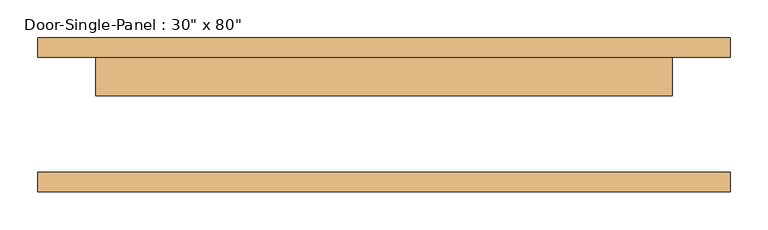
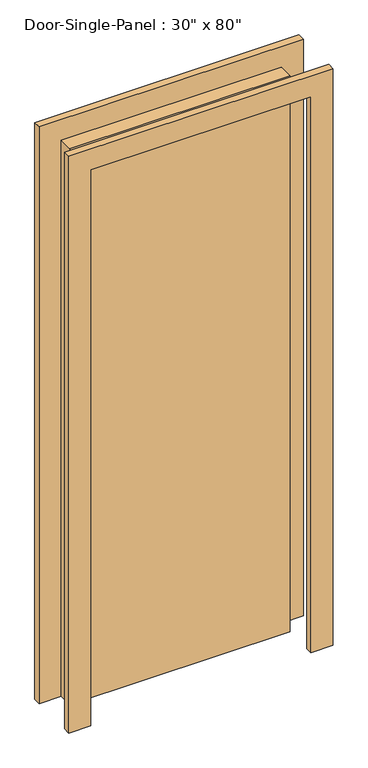
"""IFC4 building model written with IfcOpenShell, lengths in millimetres: door geometry."""

from ifc_helpers import new_model, si_unit, frame, origin, origin_with_axes, place, context, project, spatial, polyline, outline, extrude, source, transform, mapped, element, save


def door_c31ea698(model_context):
    return source(origin(), model_context, "Body", "SweptSolid", [
        extrude(outline(polyline([(381.0, 25.4), (-381.0, 25.4), (-381.0, 76.2), (381.0, 76.2), (381.0, 25.4)])), origin_with_axes(), (0.0, 0.0, 1.0), 2032.0),
        extrude(outline(polyline([(2108.2, -457.2), (0.0, -457.2), (0.0, -381.0), (2032.0, -381.0), (2032.0, 381.0), (0.0, 381.0), (0.0, 457.2), (2108.2, 457.2), (2108.2, -457.2)])), frame((0.0, 76.2, 0.0), z_axis=(0.0, 1.0, 0.0), x_axis=(0.0, 0.0, 1.0)), (0.0, 0.0, 1.0), 25.4),
        extrude(outline(polyline([(2108.2, 457.2), (2108.2, -457.2), (0.0, -457.2), (0.0, -381.0), (2032.0, -381.0), (2032.0, 381.0), (0.0, 381.0), (0.0, 457.2), (2108.2, 457.2)])), frame((0.0, -101.6, 0.0), z_axis=(0.0, 1.0, 0.0), x_axis=(0.0, 0.0, 1.0)), (0.0, 0.0, 1.0), 25.4),
    ])


if __name__ == "__main__":
    model = new_model("IFC4")
    model_context = context("Model", 3, world=origin())
    ifc_project = project(units=[si_unit("LENGTHUNIT", "METRE", prefix="MILLI")], contexts=[model_context])
    site = spatial("IfcSite", under=ifc_project)
    building = spatial("IfcBuilding", under=site)
    placement = place(None, origin())
    door_shape = door_c31ea698(model_context)
    element("IfcDoor", 1, ObjectType="Door-Single-Panel : 30\" x 80\"", at=placement, inside=building, context=model_context, shape_type="MappedRepresentation", body=[
        mapped(door_shape, transform((0.0, 0.0, 0.0), x_axis=(1.0, 0.0, 0.0), y_axis=(0.0, 1.0, 0.0), z_axis=(0.0, 0.0, 1.0))),
    ])
    save(model, "model.ifc")

# Revit data of these elements
# Type "Door-Single-Panel : 30\" x 80\""
#   Type Mark = "8"
#   Construction Type Id = "DOOR"
#   Assembly Code = "C1020300"
#   Analytic Construction = "Wooden"
#   Thickness = 0' - 2"
#   Thermal Resistance (R) = 2.5876 (h·ft²·°F)/BTU
#   Swing Angle [instance default] = 90.00°
#   Heat Transfer Coefficient (U) = 0.3865 BTU/(h·ft²·°F)
#   Height = 6' - 8"
#   Trim Projection Ext = 0' - 1"
#   Trim Projection Int = 0' - 1"
#   Trim Width = 0' - 3"
#   Width = 2' - 6"
#   Define Thermal Properties by = 1
#   Panel Material = Wood - Birch - Solid Stained Light Low Gloss
#   Trim Material = Paint - Sienna
#   Visual Light Transmittance = 0
#   Solar Heat Gain Coefficient = 0
#   Function = (empty or 0)
#   Wall Closure = (empty or 0)
# Element 1 (IfcDoor, "Door-Single-Panel : 30\" x 80\"")
#   Materials on its faces: "Paint - Sienna", "Wood - Birch - Solid Stained Light Low Gloss"
# Materials
#   "Wood - Birch - Solid Stained Light Low Gloss": class "Wood", colour RGB 210 159 95, transparency 0, Cost = 0
#   "Paint - Sienna": colour RGB 118 70 51, transparency 0, Cost = 0
